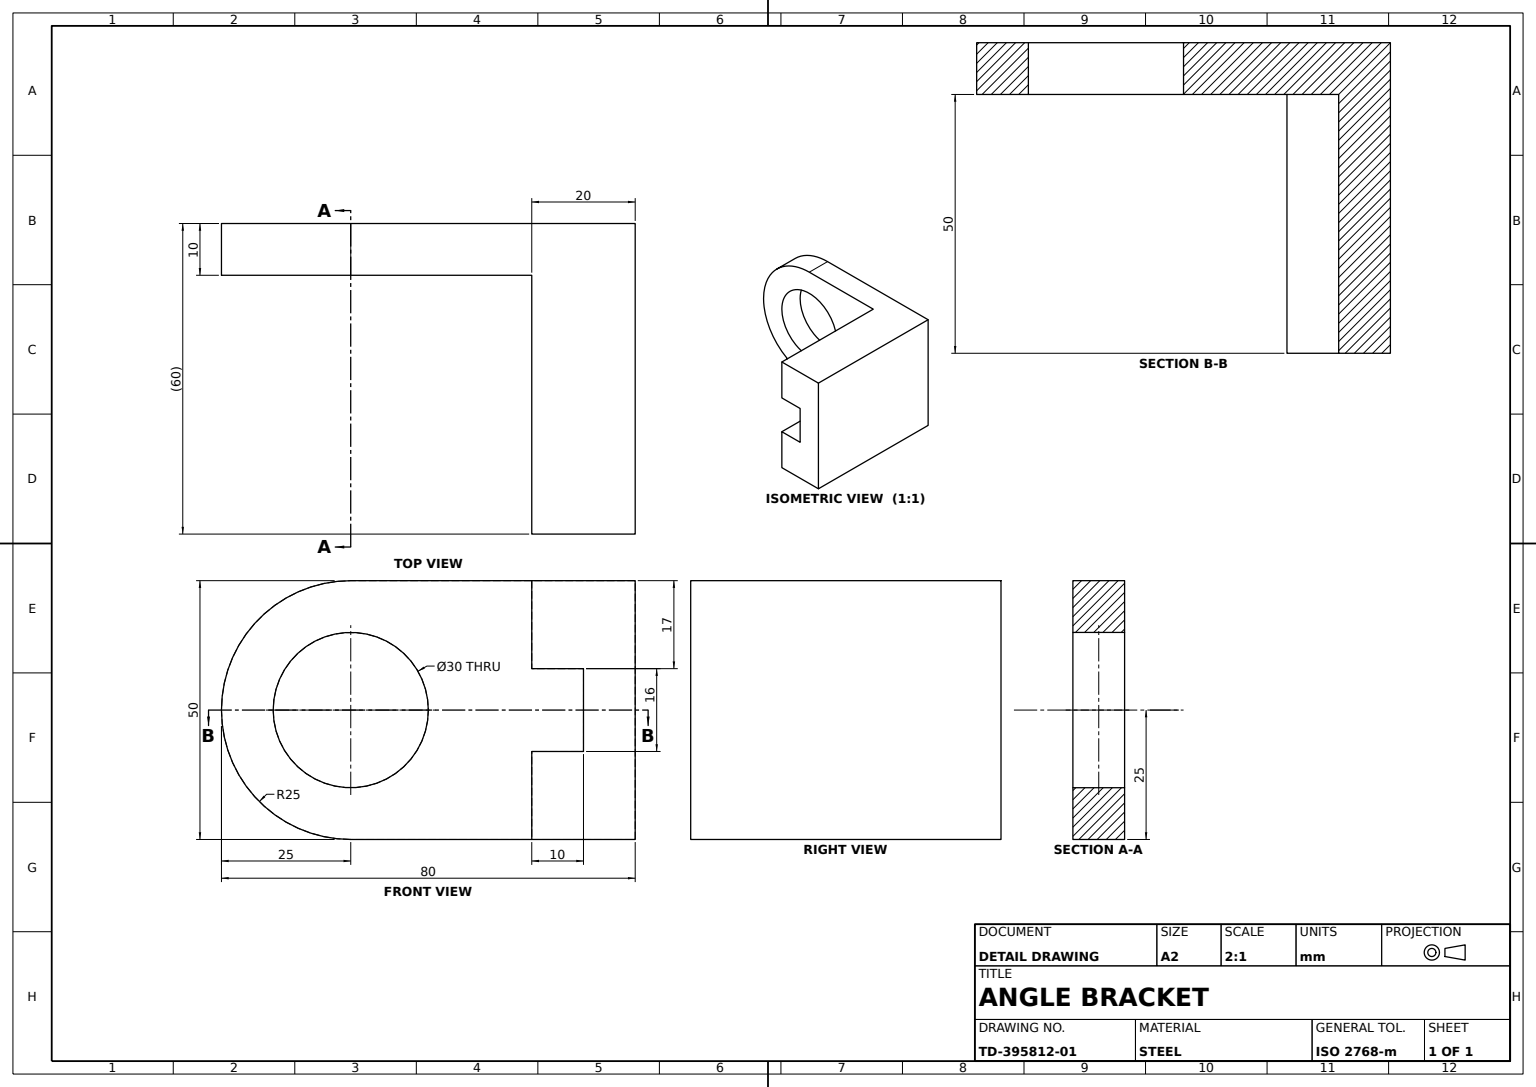
SolidWorks part; units mm, degrees
material "Plain Carbon Steel"
ref_plane "Front Plane" through (0, 0, 0) normal (0, 0, 1) x (1, 0, 0)
ref_plane "Top Plane" through (0, 0, 0) normal (0, 1, 0) x (1, 0, 0)
ref_plane "Right Plane" through (0, 0, 0) normal (1, 0, 0) x (0, 0, -1)
sketch "Base Plate Sketch" plane through (0, 0, 0) normal (0, 0, 1) x (1, 0, 0)
  line L0 (0, 0) -> (60, 0)
  line L1 (60, 0) -> (60, 50)
  line L2 (60, 50) -> (0, 50)
  line L3 (0, 50) -> (0, 0)
  dimension "D1" = 60
  dimension "D2" = 50
extrude "Base Plate" add sketch "Base Plate Sketch" along normal blind 10
sketch "Upright Block Sketch" plane through (60, 0, 0) normal (1, 0, 0) x (0, 0, -1)
  line L0 (-10, 50) -> (-20, 50)
  line L1 (-20, 50) -> (-20, 33)
  line L2 (-20, 33) -> (-10, 33)
  line L3 (-10, 0) -> (-10, 50) construction
  line L4 (-10, 33) -> (-10, 50)
  line L5 (-10, 0) -> (-20, 0)
  line L6 (-20, 0) -> (-20, 17)
  line L7 (-20, 17) -> (-10, 17)
  line L8 (-10, 17) -> (-10, 0)
  line L9 (0, 0) -> (0, 50) construction
  line L10 (-10, 50) -> (0, 50) construction
  dimension "D1" = 20
  dimension "D2" = 17
extrude "Upright Block" add sketch "Upright Block Sketch" against normal blind 60
sketch "Block Slot Sketch" plane through (0, 0, 20) normal (0, 0, 1) x (1, 0, 0)
  line L0 (0, 50) -> (10, 50)
  line L1 (0, 50) -> (60, 50) construction
  line L2 (10, 50) -> (10, 0)
  line L3 (0, 0) -> (60, 0) construction
  line L4 (10, 0) -> (0, 0)
  line L5 (0, 0) -> (0, 50)
  line L6 (60, 50) -> (60, 33) construction
  dimension "D1" = 50
extrude "Block Slot" cut sketch "Block Slot Sketch" against normal blind 10
sketch "Rounded Lug Sketch" plane through (0, 0, 0) normal (-1, 0, 0) x (0, 0, 1)
  line L0 (20, 50) -> (10, 50)
  line L1 (10, 50) -> (10, 0) construction
  line L2 (20, 50) -> (55, 50)
  line L3 (20, 0) -> (55, 0)
  line L4 (10, 50) -> (10, 0)
  line L5 (10, 0) -> (20, 0)
  arc A0 (55, 0) -> (55, 50) centre (55, 25) ccw
  dimension "D1" = 50
  dimension "D2" = 45
extrude "Rounded Lug" add sketch "Rounded Lug Sketch" against normal blind 10
sketch "Lug Hole Sketch" plane through (10, 0, 0) normal (1, 0, 0) x (0, 0, -1)
  circle A0 centre (-55, 25) radius 15
  dimension "D1" = 30
  dimension "D2" = 30
extrude "Lug Hole" cut sketch "Lug Hole Sketch" against normal blind 10
